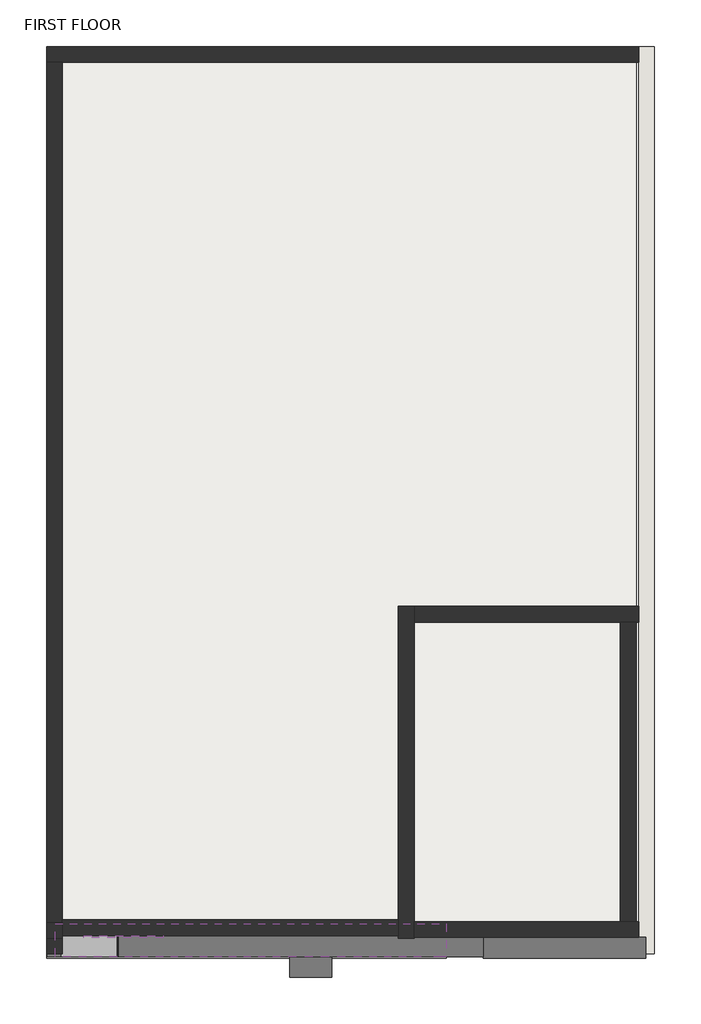
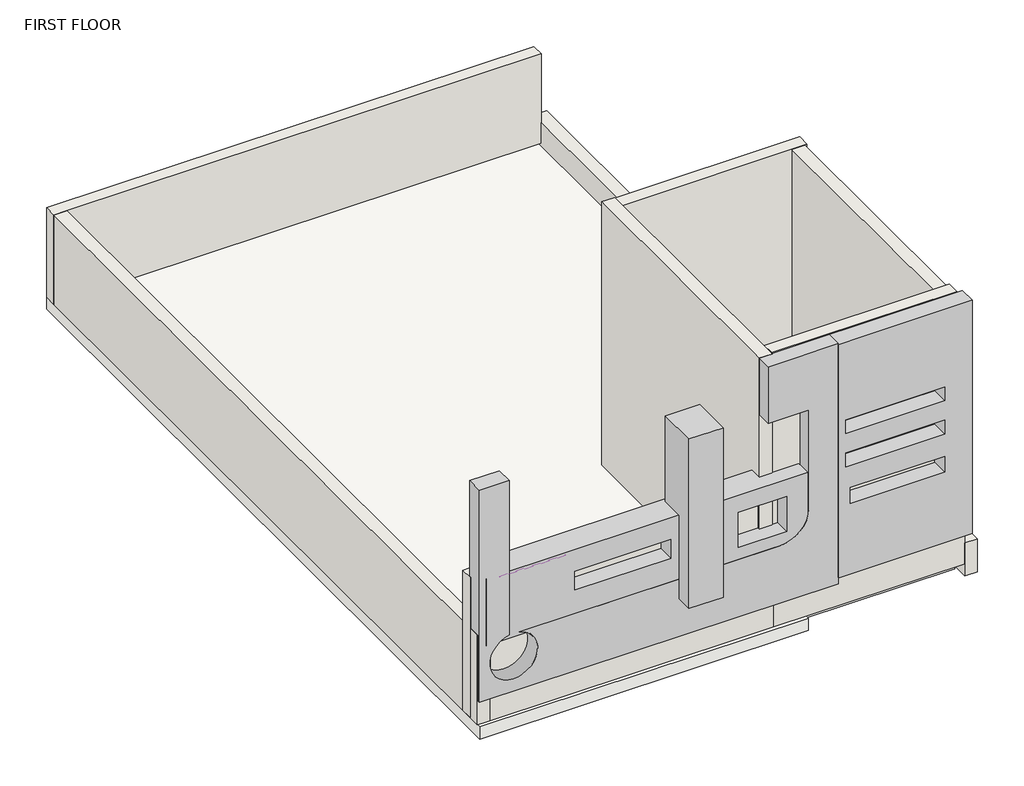
# One storey: 11 walls, 4 proxies, 1 covering, 1 slab.
"""IFC4 building model written with IfcOpenShell, lengths in millimetres."""

from ifc_helpers import new_model, si_unit, frame, origin, place, context, project, spatial, polyline, outline, extrude, faceted_brep, transform, mapped, element, save
from components import generic_models_2_generic_models_2_d1d1e900, generic_models_3_generic_models_3_4ea04a15, generic_models_4_generic_models_4_b7bd3587, generic_models_6_generic_models_6_729a5b47

model = new_model("IFC4")

# Units and contexts
model_context = context("Model", 3, world=origin())
ifc_project = project(units=[si_unit("LENGTHUNIT", "METRE", prefix="MILLI")], contexts=[model_context])

# Site, building, storey
site = spatial("IfcSite", under=ifc_project)
building = spatial("IfcBuilding", under=site)
storey = spatial("IfcBuildingStorey", under=building, Name="FIRST FLOOR", Elevation=3200.4)

# Proxies
placement = place(None, origin())
generic_models_2_generic_models_2_shape = generic_models_2_generic_models_2_d1d1e900(model_context)
element("IfcBuildingElementProxy", 1, Name="Generic Models 2 : Generic Models 2", ObjectType="Generic Models 2 : Generic Models 2", at=placement, inside=storey, context=model_context, shape_type="MappedRepresentation", body=[
    mapped(generic_models_2_generic_models_2_shape, transform((0.0, 0.0, 50.8), x_axis=(1.0, 0.0, 0.0), y_axis=(0.0, 1.0, 0.0), z_axis=(0.0, 0.0, 1.0))),
])
generic_models_3_generic_models_3_shape = generic_models_3_generic_models_3_4ea04a15(model_context)
element("IfcBuildingElementProxy", 2, Name="Generic Models 3 : Generic Models 3", ObjectType="Generic Models 3 : Generic Models 3", at=placement, inside=storey, context=model_context, shape_type="MappedRepresentation", body=[
    mapped(generic_models_3_generic_models_3_shape, transform((0.0, 0.0, 0.0), x_axis=(1.0, 0.0, 0.0), y_axis=(0.0, 1.0, 0.0), z_axis=(0.0, 0.0, 1.0))),
])
generic_models_4_generic_models_4_shape = generic_models_4_generic_models_4_b7bd3587(model_context)
element("IfcBuildingElementProxy", 3, Name="Generic Models 4 : Generic Models 4", ObjectType="Generic Models 4 : Generic Models 4", at=placement, inside=storey, context=model_context, shape_type="MappedRepresentation", body=[
    mapped(generic_models_4_generic_models_4_shape, transform((0.0, 0.0, 0.0), x_axis=(1.0, 0.0, 0.0), y_axis=(0.0, 1.0, 0.0), z_axis=(0.0, 0.0, 1.0))),
])
generic_models_6_generic_models_6_shape = generic_models_6_generic_models_6_729a5b47(model_context)
element("IfcBuildingElementProxy", 4, Name="Generic Models 6 : Generic Models 6", ObjectType="Generic Models 6 : Generic Models 6", at=placement, inside=storey, context=model_context, shape_type="MappedRepresentation", body=[
    mapped(generic_models_6_generic_models_6_shape, transform((0.0, 0.0, 0.0), x_axis=(1.0, 0.0, 0.0), y_axis=(0.0, 1.0, 0.0), z_axis=(0.0, 0.0, 1.0))),
])

# Covering
element("IfcCovering", 5, ObjectType="2' x 4' ACT System", at=placement, inside=storey, context=model_context, shape_type="SweptSolid", body=[
    extrude(outline(polyline([(-18665.6414406, -4293.1088252), (-18665.6414406, -4326.3541626), (-19829.0524212, -4326.3541626), (-19829.0524212, -4293.1088252), (-18665.6414406, -4293.1088252)])), frame((0.0, 0.0, 5638.8), z_axis=(0.0, 0.0, 1.0), x_axis=(1.0, 0.0, 0.0)), (0.0, 0.0, 1.0), 57.15),
])

# Slab
element("IfcSlab", 6, ObjectType="LW Concrete on Metal Deck", at=placement, inside=storey, context=model_context, shape_type="SweptSolid", body=[
    extrude(outline(polyline([(-11770.7356484, 8673.5911748), (-11770.7356484, -4318.5088252), (-14536.2782619, -4318.5088252), (-14536.2782619, -4623.3088252), (-20368.6358231, -4623.3088252), (-20368.6358231, 8673.5911748), (-11770.7356484, 8673.5911748)])), frame((0.0, 0.0, 2971.8), z_axis=(0.0, 0.0, 1.0), x_axis=(1.0, 0.0, 0.0)), (0.0, 0.0, 1.0), 228.6),
])

# Walls
element("IfcWall", 7, ObjectType="Generic - 9\"Masonry 2", at=placement, inside=storey, context=model_context, shape_type="Brep", body=[
    faceted_brep([(-20368.6358231, 8444.9911748, 3200.4), (-20368.6358231, -4559.8088252, 3200.4), (-20368.6358231, -4559.8088252, 4876.8), (-20368.6358231, 8444.9911748, 4876.8), (-20140.0358231, 8444.9911748, 3200.4), (-20140.0358231, 8444.9911748, 4876.8), (-20140.0358231, -4559.8088252, 4876.8), (-20140.0358231, -4559.8088252, 3769.3502296), (-20140.0358231, -4559.8088252, 3200.4), (-20140.0358231, -4331.2088252, 3200.4), (-20140.0358231, -4293.1088252, 3200.4), (-20140.0358231, -4064.5088252, 3200.4)], [[[0, 1, 2, 3]], [[4, 5, 6, 7, 8, 9, 10, 11]], [[1, 0, 4, 11, 10, 9, 8]], [[3, 2, 6, 5]], [[2, 1, 8, 7, 6]], [[0, 3, 5, 4]]]),
])
element("IfcWall", 8, ObjectType="Generic - 9\"Masonry 2", at=placement, inside=storey, context=model_context, shape_type="Brep", body=[
    faceted_brep([(-20140.0358231, -4559.8088252, 3200.4), (-15123.5356484, -4559.8088252, 3200.4), (-15123.5356484, -4559.8088252, 3769.3502296), (-15237.8356484, -4559.8088252, 3769.3502296), (-20140.0358231, -4559.8088252, 3769.3502296), (-20140.0358231, -4331.2088252, 3200.4), (-20140.0358231, -4331.2088252, 3769.3502296), (-15237.8356484, -4331.2088252, 3769.3502296), (-15123.5356484, -4331.2088252, 3769.3502296), (-15123.5356484, -4331.2088252, 3200.4), (-15237.8356484, -4331.2088252, 3200.4)], [[[0, 1, 2, 3, 4]], [[5, 6, 7, 8, 9, 10]], [[1, 0, 5, 10, 9]], [[2, 1, 9, 8]], [[4, 3, 2, 8, 7, 6]], [[0, 4, 6, 5]]]),
])
element("IfcWall", 9, ObjectType="Generic - 9\"Masonry 2", at=placement, inside=storey, context=model_context, shape_type="Brep", body=[
    faceted_brep([(-11504.0356484, -4559.8088252, 2971.8), (-11504.0356484, 8673.5911748, 2971.8), (-11504.0356484, 8673.5911748, 3589.5556148), (-11504.0356484, -4559.8088252, 3589.5556148), (-11732.6356484, -4559.8088252, 2971.8), (-11732.6356484, -4559.8088252, 3200.4), (-11732.6356484, -4559.8088252, 3589.5556148), (-11732.6356484, 8673.5911748, 3589.5556148), (-11732.6356484, 8673.5911748, 3200.4), (-11732.6356484, 8673.5911748, 2971.8)], [[[0, 1, 2, 3]], [[4, 5, 6, 7, 8, 9]], [[1, 0, 4, 9]], [[3, 2, 7, 6]], [[2, 1, 9, 8, 7]], [[0, 3, 6, 5, 4]]]),
])
element("IfcWall", 10, ObjectType="Generic - 9\"Masonry 2", at=placement, inside=storey, context=model_context, shape_type="Brep", body=[
    faceted_brep([(-11732.6356484, 8673.5911748, 3200.4), (-20368.6358231, 8673.5911748, 3200.4), (-20368.6358231, 8673.5911748, 4876.8), (-11732.6356484, 8673.5911748, 4876.8), (-11732.6356484, 8673.5911748, 3589.5556148), (-11732.6356484, 8444.9911748, 3200.4), (-11732.6356484, 8444.9911748, 4876.8), (-20140.0358231, 8444.9911748, 4876.8), (-20368.6358231, 8444.9911748, 4876.8), (-20368.6358231, 8444.9911748, 3200.4), (-20140.0358231, 8444.9911748, 3200.4)], [[[0, 1, 2, 3, 4]], [[5, 6, 7, 8, 9, 10]], [[1, 0, 5, 10, 9]], [[3, 2, 8, 7, 6]], [[0, 4, 3, 6, 5]], [[2, 1, 9, 8]]]),
])
element("IfcWall", 11, ObjectType="Generic - 9\"Masonry 2", at=placement, inside=storey, context=model_context, shape_type="Brep", body=[
    faceted_brep([(-15123.5356484, -4559.8088252, 3200.4), (-11732.6356484, -4559.8088252, 3200.4), (-11732.6356484, -4559.8088252, 3589.5556148), (-11732.6356484, -4559.8088252, 3813.1326905), (-15237.8356484, -4559.8088252, 3813.1326905), (-15237.8356484, -4559.8088252, 3769.3502296), (-15123.5356484, -4559.8088252, 3769.3502296), (-15123.5356484, -4331.2088252, 3200.4), (-15123.5356484, -4331.2088252, 3769.3502296), (-15237.8356484, -4331.2088252, 3769.3502296), (-15237.8356484, -4331.2088252, 3813.1326905), (-11732.6356484, -4331.2088252, 3813.1326905), (-11732.6356484, -4331.2088252, 3200.4), (-15009.2356484, -4331.2088252, 3200.4)], [[[0, 1, 2, 3, 4, 5, 6]], [[7, 8, 9, 10, 11, 12, 13]], [[1, 0, 7, 13, 12]], [[4, 3, 11, 10]], [[3, 2, 1, 12, 11]], [[0, 6, 8, 7]], [[5, 9, 8, 6]], [[5, 4, 10, 9]]]),
])
element("IfcWall", 12, ObjectType="Generic - 9\"Masonry 2", at=placement, inside=storey, context=model_context, shape_type="Brep", body=[
    faceted_brep([(-15237.8356484, 507.4911748, 3200.4), (-15237.8356484, -4064.5088252, 3200.4), (-15237.8356484, -4293.1088252, 3200.4), (-15237.8356484, -4331.2088252, 3200.4), (-15237.8356484, -4331.2088252, 3769.3502296), (-15237.8356484, -4331.2088252, 3813.1326905), (-15237.8356484, -4331.2088252, 8144.858524), (-15237.8356484, 507.4911748, 8144.858524), (-15009.2356484, 507.4911748, 3200.4), (-15009.2356484, 507.4911748, 8134.0226581), (-15009.2356484, 507.4911748, 8144.858524), (-15009.2356484, -4331.2088252, 8144.858524), (-15009.2356484, -4331.2088252, 3200.4), (-15009.2356484, -4318.5088252, 3200.4), (-15009.2356484, -4089.9088252, 3200.4), (-15009.2356484, 278.8911748, 3200.4), (-15123.5356484, -4331.2088252, 3200.4)], [[[0, 1, 2, 3, 4, 5, 6, 7]], [[8, 9, 10, 11, 12, 13, 14, 15]], [[3, 2, 1, 0, 8, 15, 14, 13, 12, 16]], [[7, 6, 11, 10]], [[0, 7, 10, 9, 8]], [[3, 16, 12, 11, 6, 5, 4]]]),
])
element("IfcWall", 13, ObjectType="Generic - 9\"Masonry 2", at=placement, inside=storey, context=model_context, shape_type="Brep", body=[
    faceted_brep([(-15009.2356484, 278.8911748, 3200.4), (-11999.3356484, 278.8911748, 3200.4), (-11770.7356484, 278.8911748, 3200.4), (-11732.6356484, 278.8911748, 3200.4), (-11732.6356484, 278.8911748, 8134.0226581), (-15009.2356484, 278.8911748, 8134.0226581), (-15009.2356484, 507.4911748, 3200.4), (-15009.2356484, 507.4911748, 8134.0226581), (-11732.6356484, 507.4911748, 8134.0226581), (-11732.6356484, 507.4911748, 3200.4)], [[[0, 1, 2, 3, 4, 5]], [[6, 7, 8, 9]], [[3, 2, 1, 0, 6, 9]], [[5, 4, 8, 7]], [[0, 5, 7, 6]], [[4, 3, 9, 8]]]),
])
element("IfcWall", 14, ObjectType="Generic - 9\"Masonry 2", at=placement, inside=storey, context=model_context, shape_type="Brep", body=[
    faceted_brep([(-15009.2356484, -4318.5088252, 3200.4), (-11732.6356484, -4318.5088252, 3200.4), (-11732.6356484, -4318.5088252, 8159.197303), (-15009.2356484, -4318.5088252, 8159.197303), (-15009.2356484, -4089.9088252, 3200.4), (-15009.2356484, -4089.9088252, 8159.197303), (-11732.6356484, -4089.9088252, 8159.197303), (-11732.6356484, -4089.9088252, 3200.4), (-11770.7356484, -4089.9088252, 3200.4), (-11999.3356484, -4089.9088252, 3200.4)], [[[0, 1, 2, 3]], [[4, 5, 6, 7, 8, 9]], [[1, 0, 4, 9, 8, 7]], [[3, 2, 6, 5]], [[2, 1, 7, 6]], [[0, 3, 5, 4]]]),
])
element("IfcWall", 15, ObjectType="Generic - 9\"Masonry 2", at=placement, inside=storey, context=model_context, shape_type="SweptSolid", body=[
    extrude(outline(polyline([(-11770.7356484, 278.8911748), (-11770.7356484, -4089.9088252), (-11999.3356484, -4089.9088252), (-11999.3356484, 278.8911748), (-11770.7356484, 278.8911748)])), frame((0.0, 0.0, 3200.4), z_axis=(0.0, 0.0, 1.0), x_axis=(1.0, 0.0, 0.0)), (0.0, 0.0, 1.0), 4928.7297902),
])
element("IfcWall", 16, ObjectType="Generic - 9\"Masonry 2", at=placement, inside=storey, context=model_context, shape_type="SweptSolid", body=[
    extrude(outline(polyline([(-15237.8356484, -4293.1088252), (-20140.0358231, -4293.1088252), (-20140.0358231, -4064.5088252), (-15237.8356484, -4064.5088252), (-15237.8356484, -4293.1088252)])), frame((0.0, 0.0, 3200.4), z_axis=(0.0, 0.0, 1.0), x_axis=(1.0, 0.0, 0.0)), (0.0, 0.0, 1.0), 2608.6263876),
])
element("IfcWall", 17, ObjectType="Generic - 9\"Masonry 2", at=placement, inside=storey, context=model_context, shape_type="SweptSolid", body=[
    extrude(outline(polyline([(-20368.6358231, -4102.6088252), (-20140.0358231, -4102.6088252), (-20140.0358231, -4331.2088252), (-20368.6358231, -4331.2088252), (-20368.6358231, -4102.6088252)])), frame((0.0, 0.0, 3200.4), z_axis=(0.0, 0.0, 1.0), x_axis=(1.0, 0.0, 0.0)), (0.0, 0.0, 1.0), 2625.0969172),
])

save(model, "model.ifc")

# Revit data of these elements
# Type "2' x 4' ACT System"
#   Assembly Code = "C3030210"
#   built-in parameter 1002203 = 1 (stored number, unit not read)
#   built-in parameter 1002202 = 1 (stored number, unit not read)
#   Layers, outside or top first: 0' - 1 5/8" "Default" (function 1); 0' - 0 5/8" "Acoustic Ceiling Tile 24 x 48" (function 5)
# Type "LW Concrete on Metal Deck"
#   Assembly Code = "B1010"
#   Function = 0
#   Layers, outside or top first: 0' - 4" "Concrete, Lightweight" (function 1); 0' - 5" "Metal Deck" (function 1)
# Type "Generic - 9\"Masonry 2"
#   Assembly Code = "B2010"
#   Layers, outside or top first: 0' - 9" "Concrete Masonry Units" (function 1)
# Element 1 (IfcBuildingElementProxy, "Generic Models 2 : Generic Models 2")
#   Phase Created = New Construction
# Element 2 (IfcBuildingElementProxy, "Generic Models 3 : Generic Models 3")
#   Phase Created = New Construction
# Element 3 (IfcBuildingElementProxy, "Generic Models 4 : Generic Models 4")
#   Phase Created = New Construction
# Element 4 (IfcBuildingElementProxy, "Generic Models 6 : Generic Models 6")
#   Phase Created = New Construction
# Element 5 (IfcCovering, "2' x 4' ACT System")
#   Height Offset From Level = 8' - 0"
#   Phase Created = New Construction
#   Materials on its faces: "Acoustic Ceiling Tile 24 x 48", "Default"
# Element 6 (IfcSlab, "LW Concrete on Metal Deck")
#   Height Offset From Level = 0' - 0"
#   Phase Created = New Construction
#   Materials on its faces: "Metal Deck", "Concrete, Lightweight"
# Elements 7, 10 (IfcWall, "Generic - 9\"Masonry 2")
#   Top Offset = -0' - 6"
#   Base Offset = 0' - 0"
#   wall height = 5' - 6"
#   Phase Created = New Construction
#   Base Constraint = FIRST FLOOR
#   Top Constraint = parapet wall
#   Materials on its faces: "Concrete Masonry Units"
# Element 8 (IfcWall, "Generic - 9\"Masonry 2")
#   Top Offset = -4' - 1.60038"
#   Base Offset = 0' - 0"
#   wall height = 1' - 10.39962"
#   Phase Created = New Construction
#   Base Constraint = FIRST FLOOR
#   Top Constraint = parapet wall
#   Materials on its faces: "Concrete Masonry Units"
# Element 9 (IfcWall, "Generic - 9\"Masonry 2")
#   built-in parameter 1001111 = -0' - 9"
#   Top Offset = -4' - 8.67891"
#   Base Offset = -0' - 9"
#   wall height = 2' - 0.32109"
#   Phase Created = New Construction
#   Base Constraint = FIRST FLOOR
#   Top Constraint = parapet wall
#   Materials on its faces: "Concrete Masonry Units"
# Element 11 (IfcWall, "Generic - 9\"Masonry 2")
#   Top Offset = -3' - 11.87667"
#   Base Offset = 0' - 0"
#   wall height = 2' - 0.12333"
#   Phase Created = New Construction
#   Base Constraint = FIRST FLOOR
#   Top Constraint = parapet wall
#   Materials on its faces: "Concrete Masonry Units"
# Element 12 (IfcWall, "Generic - 9\"Masonry 2")
#   Top Offset = 0' - 0"
#   Base Offset = 0' - 0"
#   Unconnected Height = 16' - 2.66372"
#   wall height = 16' - 2.66372"
#   Phase Created = New Construction
#   Base Constraint = FIRST FLOOR
#   Materials on its faces: "Concrete Masonry Units"
# Element 13 (IfcWall, "Generic - 9\"Masonry 2")
#   Top Offset = 0' - 0"
#   Base Offset = 0' - 0"
#   Unconnected Height = 16' - 2.23711"
#   wall height = 16' - 2.23711"
#   Phase Created = New Construction
#   Base Constraint = FIRST FLOOR
#   Materials on its faces: "Concrete Masonry Units"
# Element 14 (IfcWall, "Generic - 9\"Masonry 2")
#   Top Offset = 10' - 3.22824"
#   Base Offset = 0' - 0"
#   wall height = 16' - 3.22824"
#   Phase Created = New Construction
#   Base Constraint = FIRST FLOOR
#   Top Constraint = parapet wall
#   Materials on its faces: "Concrete Masonry Units"
# Element 15 (IfcWall, "Generic - 9\"Masonry 2")
#   Top Offset = 0' - 0"
#   Base Offset = 0' - 0"
#   Unconnected Height = 16' - 2.04448"
#   wall height = 16' - 2.04448"
#   Phase Created = New Construction
#   Base Constraint = FIRST FLOOR
#   Materials on its faces: "Concrete Masonry Units"
# Element 16 (IfcWall, "Generic - 9\"Masonry 2")
#   Top Offset = 0' - 0"
#   Base Offset = 0' - 0"
#   Unconnected Height = 8' - 6.70183"
#   wall height = 8' - 6.70183"
#   Phase Created = New Construction
#   Base Constraint = FIRST FLOOR
#   Materials on its faces: "Concrete Masonry Units"
# Element 17 (IfcWall, "Generic - 9\"Masonry 2")
#   Top Offset = 0' - 0"
#   Base Offset = 0' - 0"
#   Unconnected Height = 8' - 7.35027"
#   wall height = 8' - 7.35027"
#   Phase Created = New Construction
#   Base Constraint = FIRST FLOOR
#   Materials on its faces: "Concrete Masonry Units"
# Materials
#   "Default": colour RGB 127 127 127, transparency 0, Cost = 0
#   "Acoustic Ceiling Tile 24 x 48": class "Generic", colour RGB 229 229 229, transparency 0, Description = "Acoustic Ceiling Tile 24 x 48", Cost = 0
#   "Concrete, Lightweight": class "Concrete", colour RGB 142 141 140, transparency 0, Description = "Lightweight concrete", Cost = 0
#   "Metal Deck": class "Metal", colour RGB 199 199 199, transparency 0, Description = "Steel, mill finish", Cost = 0
#   "Concrete Masonry Units": class "Masonry", colour RGB 227 227 227, transparency 0, Description = "Concrete masonry units", Cost = 0
